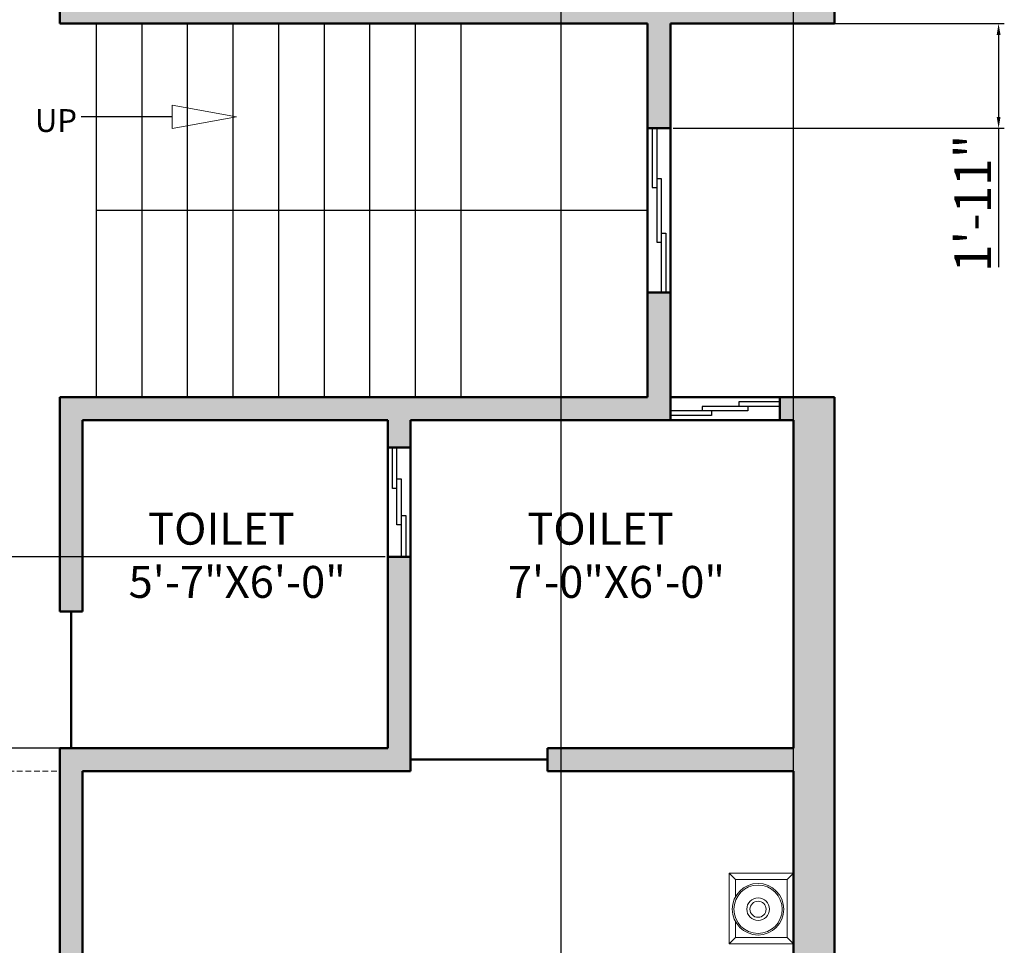
# Model space of a CAD drawing. Units: inches. Extents: x 1913 to 5309, y 1003 to 1733.
# Tile 20 of 23: x 4336 to 4552, y 1286 to 1489. Entities that reach past the tile are written whole.
import ezdxf

# ---------------------------------------------------------------- set-up
doc = ezdxf.new("R2010")
doc.units = ezdxf.units.IN
doc.linetypes.add('HIDDEN2', pattern=[0.1875, 0.125, -0.0625])
for name, color, linetype, lineweight in [('0.15', 34, 'Continuous', 15), ('A-ANNO-DIMS', 2, 'Continuous', 18), ('A-ANNO-SYMB', 1, 'Continuous', 18), ('A-ANNO-TEXT', 7, 'Continuous', 18), ('A-AREA-IDEN', 3, 'Continuous', 18), ('A-FLOR-PATT', 252, 'Continuous', 13), ('A-FLOR-STRS', 7, 'Continuous', 25), ('A-FURN', 8, 'Continuous', 18), ('A-GLAZ', 5, 'Continuous', 25), ('A-WALL', 7, 'Continuous', 50), ('A-WALL-OVHD', 8, 'HIDDEN2', 18)]:
    doc.layers.add(name, color=color, linetype=linetype, lineweight=lineweight)
doc.styles.get("Standard").update_dxf_attribs({"font": 'arial.ttf'})
doc.dimstyles.new('ISO-25', dxfattribs={"dimtxt": 8, "dimasz": 2.5, "dimexe": 1.25, "dimexo": 0.625, "dimtad": 1, "dimdec": 1, "dimlunit": 3, "dimtxsty": 'Standard', "dimcen": 2.5, "dimclrd": 256, "dimclrt": 1, "dimadec": 0, "dimazin": 0, "dimtfac": 1, "dimtdec": 1, "dimtmove": 0, "dimatfit": 3, "dimfxl": 1, "dimarcsym": 0})

# ---------------------------------------------------------------- blocks, each defined once
blk = doc.blocks.new('VELADOR')
at = {"layer": '0.15'}
for p, q in [((-0.2475, 0), (-0.2025, -0.045)), ((0.2475, 0), (0.2025, -0.045)), ((-0.2025, -0.405), (-0.2475, -0.45)), ((0.2475, -0.45), (0.2025, -0.405))]:
    blk.add_line(p, q, dxfattribs=at)
blk.add_lwpolyline([(-0.2475, 0), (-0.2475, -0.45), (0.2475, -0.45), (0.2475, 0)], close=True, dxfattribs=at)
blk.add_lwpolyline([(0.0921, -0.405), (0.2025, -0.405), (0.2025, -0.045), (-0.2025, -0.045), (-0.2025, -0.405), (-0.0818, -0.405)], dxfattribs=at)
for radius in [0.18, 0.1688, 0.0788, 0.0563]:
    blk.add_circle((0.0052, -0.2474), radius, dxfattribs=at)
blk = doc.blocks.new('WIN-24')
for p, q in [((0, 15), (0, 24)), ((1, 7), (1, 24)), ((2, 17), (1, 17)), ((2, 0), (2, 17)), ((1, 15), (0, 15)), ((3, 9), (2, 9)), ((3, 0), (3, 9)), ((2, 7), (1, 7))]:
    blk.add_line(p, q)
blk = doc.blocks.new('WIN-36')
for p, q in [((0, 23), (0, 36)), ((1, 11), (1, 36)), ((2, 25), (1, 25)), ((2, 0), (2, 25)), ((1, 23), (0, 23)), ((3, 13), (2, 13)), ((3, 0), (3, 13)), ((2, 11), (1, 11))]:
    blk.add_line(p, q)
blk = doc.blocks.new('*D110')
at = {"layer": 'A-ANNO-DIMS', "color": 0, "lineweight": -2, "transparency": 16777216}
for p, q in [((4479.84, 1487.96), (4552.46, 1487.96)), ((4479.84, 1464.96), (4552.46, 1464.96))]:
    blk.add_line(p, q, dxfattribs=at)
at = {"layer": 'A-ANNO-DIMS', "lineweight": -2, "transparency": 16777216}
for p, q in [((4551.21, 1485.46), (4551.21, 1467.46)), ((4551.21, 1464.96), (4551.21, 1434.49))]:
    blk.add_line(p, q, dxfattribs=at)
at = {"layer": 'A-ANNO-DIMS', "transparency": 16777216}
for points in [[(4550.8, 1485.46), (4551.63, 1485.46), (4551.21, 1487.96)], [(4550.8, 1467.46), (4551.63, 1467.46), (4551.21, 1464.96)]]:
    blk.add_solid(points, dxfattribs=at)
at = {"layer": 'Defpoints', "color": 0, "transparency": 16777216}
for p in [(4479.21, 1487.96), (4479.21, 1464.96), (4551.21, 1464.96)]:
    blk.add_point(p, dxfattribs=at)
at = {"layer": 'A-ANNO-DIMS', "color": 1, "transparency": 16777216, "insert": (4546.57, 1448.47), "char_height": 8, "attachment_point": 5, "rotation": 90}
blk.add_mtext('1\'-11"', dxfattribs=at)
blk = doc.blocks.new('*D113')
at = {"layer": 'A-ANNO-DIMS', "color": 0, "lineweight": -2, "transparency": 16777216}
for p, q in [((4455.21, 1180.59), (4455.21, 1724.21)), ((4506.21, 1180.59), (4506.21, 1724.21))]:
    blk.add_line(p, q, dxfattribs=at)
at = {"layer": 'A-ANNO-DIMS', "lineweight": -2, "transparency": 16777216}
blk.add_line((4457.71, 1722.96), (4503.71, 1722.96), dxfattribs=at)
at = {"layer": 'A-ANNO-DIMS', "transparency": 16777216}
for points in [[(4457.71, 1723.38), (4457.71, 1722.55), (4455.21, 1722.96)], [(4503.71, 1723.38), (4503.71, 1722.55), (4506.21, 1722.96)]]:
    blk.add_solid(points, dxfattribs=at)
at = {"layer": 'Defpoints', "color": 0, "transparency": 16777216}
for p in [(4506.21, 1722.96), (4455.21, 1179.96), (4506.21, 1179.96)]:
    blk.add_point(p, dxfattribs=at)
at = {"layer": 'A-ANNO-DIMS', "color": 1, "transparency": 16777216, "insert": (4480.71, 1727.68), "char_height": 8, "attachment_point": 5}
blk.add_mtext('4\'-3"', dxfattribs=at)
blk = doc.blocks.new('*D115')
at = {"layer": 'A-ANNO-DIMS', "color": 0, "lineweight": -2, "transparency": 16777216}
for p, q in [((4416.59, 1370.96), (3925.96, 1370.96)), ((4416.59, 1328.96), (3925.96, 1328.96))]:
    blk.add_line(p, q, dxfattribs=at)
at = {"layer": 'A-ANNO-DIMS', "lineweight": -2, "transparency": 16777216}
blk.add_line((3927.21, 1331.46), (3927.21, 1368.46), dxfattribs=at)
at = {"layer": 'A-ANNO-DIMS', "transparency": 16777216}
for points in [[(3926.8, 1368.46), (3927.63, 1368.46), (3927.21, 1370.96)], [(3926.8, 1331.46), (3927.63, 1331.46), (3927.21, 1328.96)]]:
    blk.add_solid(points, dxfattribs=at)
at = {"layer": 'Defpoints', "color": 0, "transparency": 16777216}
for p in [(3927.21, 1370.96), (4417.21, 1370.96), (4417.21, 1328.96)]:
    blk.add_point(p, dxfattribs=at)
at = {"layer": 'A-ANNO-DIMS', "color": 1, "transparency": 16777216, "insert": (3922.5, 1349.96), "char_height": 8, "attachment_point": 5, "rotation": 90}
blk.add_mtext('3\'-6"', dxfattribs=at)

msp = doc.modelspace()

# ---------------------------------------------------------------- hatches: boundary and pattern name
at = {"layer": 'A-FLOR-PATT'}
h = msp.add_hatch(color=256, dxfattribs=at)
h.dxf.hatch_style = 1
h.paths.add_polyline_path([(4179.21, 1155.93), (4164.35, 1155.93, -0.035946), (4163.9, 1155.96), (4161.21, 1155.96), (4161.21, 1173.96), (4152.21, 1173.96), (4152.21, 1146.96), (4179.21, 1146.96)])
h.paths.add_polyline_path([(4273.21, 1155.96), (4266.93, 1155.96), (4233.21, 1155.96), (4233.21, 1146.96), (4273.21, 1146.96)])
h.paths.add_polyline_path([(4285.21, 1328.96), (4152.21, 1328.96), (4152.21, 1305.96), (4161.21, 1305.96), (4161.21, 1323.96), (4285.21, 1323.96)])
h.paths.add_polyline_path([(4161.21, 1257.96), (4152.21, 1257.96), (4152.21, 1233.96), (4161.21, 1233.96), (4161.21, 1237.71)])
h.paths.add_polyline_path([(4515.21, 1405.96), (4503.21, 1405.96), (4503.21, 1400.96), (4506.21, 1400.96), (4506.21, 1328.96), (4452.21, 1328.96), (4452.21, 1323.96), (4506.21, 1323.96), (4506.21, 1179.96), (4455.21, 1179.96), (4455.21, 1170.96), (4515.21, 1170.96)])
h.paths.add_polyline_path([(4157.21, 1686.96), (3999.21, 1686.96), (3999.21, 1625.96), (4008.21, 1625.96), (4008.21, 1677.96), (4152.21, 1677.96), (4152.21, 1554.96), (4157.21, 1554.96), (4157.21, 1599.96), (4225.21, 1599.96), (4225.21, 1608.96), (4157.21, 1608.96)])
h.paths.add_polyline_path([(4008.21, 1513.96), (4157.21, 1513.96), (4157.21, 1518.96), (4008.21, 1518.96), (4008.21, 1571.96), (3999.21, 1571.96), (3999.21, 1420.96), (4050.21, 1420.96), (4050.21, 1429.96), (4008.21, 1429.96)])
h.paths.add_polyline_path([(4157.21, 1477.96), (4152.21, 1477.96), (4152.21, 1429.96), (4110.21, 1429.96), (4110.21, 1420.96), (4157.21, 1420.96)], flags=17)
h.paths.add_polyline_path([(4350.21, 1608.96), (4345.21, 1608.96), (4321.21, 1608.96), (4321.21, 1599.96), (4350.21, 1599.96)])
h.paths.add_polyline_path([(4515.21, 1686.96), (4345.21, 1686.96), (4345.21, 1644.96), (4350.21, 1644.96), (4350.21, 1677.96), (4506.21, 1677.96), (4506.21, 1557.96), (4423.21, 1557.96), (4423.21, 1552.96), (4506.21, 1552.96), (4506.21, 1492.96), (4428.21, 1492.96), (4428.21, 1522.96), (4423.21, 1522.96), (4423.21, 1492.96), (4345.21, 1492.96), (4345.21, 1487.96), (4474.21, 1487.96), (4474.21, 1464.96), (4479.21, 1464.96), (4479.21, 1487.96), (4515.21, 1487.96)])
h.paths.add_polyline_path([(4479.21, 1428.96), (4474.21, 1428.96), (4474.21, 1405.96), (4345.21, 1405.96), (4345.21, 1358.96), (4350.21, 1358.96), (4350.21, 1400.96), (4417.21, 1400.96), (4417.21, 1394.96), (4422.21, 1394.96), (4422.21, 1400.96), (4479.21, 1400.96)])
h.paths.add_polyline_path([(4350.21, 1323.96), (4422.21, 1323.96), (4422.21, 1370.96), (4417.21, 1370.96), (4417.21, 1328.96), (4345.21, 1328.96), (4345.21, 1158.97, -0.414214), (4342.21, 1155.96), (4327.21, 1155.96), (4327.21, 1146.96), (4350.21, 1146.96), (4350.21, 1170.96), (4401.21, 1170.96), (4401.21, 1179.96), (4350.21, 1179.96)])
h.paths.add_polyline_path([(4157.21, 1356.96), (4152.21, 1356.96), (4152.21, 1352.96), (4157.21, 1352.96)])
h.paths.add_polyline_path([(4157.21, 1396.96), (4152.21, 1396.96), (4152.21, 1392.96), (4157.21, 1392.96)])

# ---------------------------------------------------------------- linework, layer by layer
at = {"layer": 'A-ANNO-SYMB'}
msp.add_lwpolyline([(4384.04, 1467.46), (4369.88, 1470.02), (4369.88, 1464.91)], close=True, dxfattribs=at)
at = {"layer": 'A-FLOR-STRS'}
for p, q in [((4353.21, 1487.96), (4353.21, 1405.96)), ((4363.21, 1487.96), (4363.21, 1405.96)), ((4373.21, 1487.96), (4373.21, 1405.96)), ((4383.21, 1487.96), (4383.21, 1405.96)), ((4393.21, 1487.96), (4393.21, 1405.96)), ((4403.21, 1487.96), (4403.21, 1405.96)), ((4413.21, 1487.96), (4413.21, 1405.96)), ((4423.21, 1487.96), (4423.21, 1405.96)), ((4433.21, 1487.96), (4433.21, 1405.96)), ((4369.88, 1467.46), (4349.96, 1467.46)), ((4474.21, 1446.96), (4353.21, 1446.96))]:
    msp.add_line(p, q, dxfattribs=at)
at = {"layer": 'A-WALL'}
for p, q in [((4515.21, 1686.96), (4515.21, 1487.96)), ((4345.21, 1492.96), (4345.21, 1487.96)), ((4345.21, 1487.96), (4474.21, 1487.96)), ((4474.21, 1487.96), (4474.21, 1405.96)), ((4479.21, 1487.96), (4479.21, 1400.96)), ((4479.21, 1487.96), (4515.21, 1487.96)), ((4479.21, 1464.96), (4474.21, 1464.96)), ((4479.21, 1428.96), (4474.21, 1428.96)), ((4345.21, 1405.96), (4474.21, 1405.96)), ((4345.21, 1405.96), (4345.21, 1358.96)), ((4479.21, 1405.96), (4515.21, 1405.96)), ((4503.21, 1405.96), (4503.21, 1400.96)), ((4515.21, 1405.96), (4515.21, 1098.96)), ((4350.21, 1400.96), (4350.21, 1358.96)), ((4350.21, 1400.96), (4417.21, 1400.96)), ((4417.21, 1400.96), (4417.21, 1328.96)), ((4422.21, 1400.96), (4422.21, 1323.96)), ((4422.21, 1400.96), (4506.21, 1400.96)), ((4506.21, 1400.96), (4506.21, 1328.96)), ((4417.21, 1394.96), (4422.21, 1394.96)), ((4417.21, 1370.96), (4422.21, 1370.96)), ((4345.21, 1358.96), (4350.21, 1358.96)), ((4347.71, 1358.96), (4347.71, 1328.96)), ((4345.21, 1328.96), (4345.21, 1155.96)), ((4345.21, 1328.96), (4417.21, 1328.96)), ((4452.21, 1328.96), (4506.21, 1328.96)), ((4452.21, 1328.96), (4452.21, 1323.96)), ((4452.21, 1326.46), (4422.21, 1326.46)), ((4350.21, 1323.96), (4350.21, 1179.96)), ((4350.21, 1323.96), (4422.21, 1323.96)), ((4452.21, 1323.96), (4506.21, 1323.96)), ((4506.21, 1323.96), (4506.21, 1179.96))]:
    msp.add_line(p, q, dxfattribs=at)
at = {"layer": 'A-WALL-OVHD', "ltscale": 10}
for p, q in [((4285.21, 1328.96), (4345.21, 1328.96)), ((4285.21, 1323.96), (4345.21, 1323.96))]:
    msp.add_line(p, q, dxfattribs=at)

# ---------------------------------------------------------------- block references
at = {"layer": 'A-FURN', "xscale": 31.41542173157097, "yscale": 31.41542173157097, "zscale": 31.41542173157097, "rotation": 270}
msp.add_blockref('VELADOR', (4506.21, 1293.8), dxfattribs=at)
at = {"layer": 'A-GLAZ'}
for name, p, rotation in [('WIN-36', (4478.21, 1464.96), 180), ('WIN-24', (4503.21, 1401.96), 89.99999999999213)]:
    msp.add_blockref(name, p, dxfattribs=dict(at, rotation=rotation))
msp.add_blockref('WIN-24', (4418.21, 1370.96), dxfattribs=at)

# ---------------------------------------------------------------- texts
at = {"layer": 'A-ANNO-TEXT', "insert": (4339.77, 1469.16), "char_height": 5, "attachment_point": 1}
msp.add_mtext_dynamic_manual_height_columns('{UP}', width=10.7355, gutter_width=12.5, heights=[0], dxfattribs=at)
at = {"layer": 'A-AREA-IDEN', "char_height": 7, "attachment_point": 1}
for s, insert in [('  TOILET\\P5\'-7"X6\'-0"', (4360.33, 1380.62)), ('  TOILET\\P7\'-0"X6\'-0"', (4443.53, 1380.62))]:
    msp.add_mtext_dynamic_manual_height_columns(s, width=86.9528, gutter_width=12.5, heights=[0], dxfattribs=dict(at, insert=insert))

# ---------------------------------------------------------------- dimensions: what is measured, and where the dimension line sits
at = {"layer": 'A-ANNO-DIMS'}
dim = msp.add_linear_dim(base=(4506.21, 1722.96), p1=(4455.21, 1179.96), p2=(4506.21, 1179.96), dimstyle='ISO-25', override={"dimdec": 1, "dimlfac": 1, "dimrnd": 0, "dimzin": 1, "dimdsep": 46, "dimlunit": 4, "dimfrac": 2}, dxfattribs=at)
dim.commit()
dim.dimension.update_dxf_attribs({"geometry": '*D113', "text_midpoint": (4480.71, 1727.68)})
for base, p1, p2, picture, middle in [((4551.21, 1464.96), (4479.21, 1487.96), (4479.21, 1464.96), '*D110', (4546.57, 1448.47)), ((3927.21, 1370.96), (4417.21, 1328.96), (4417.21, 1370.96), '*D115', (3922.5, 1349.96))]:
    dim = msp.add_linear_dim(base=base, p1=p1, p2=p2, angle=90, dimstyle='ISO-25', override={"dimdec": 1, "dimlfac": 1, "dimrnd": 0, "dimzin": 1, "dimdsep": 46, "dimlunit": 4, "dimfrac": 2}, dxfattribs=at)
    dim.commit()
    dim.dimension.update_dxf_attribs({"geometry": picture, "text_midpoint": middle})

doc.saveas('drawing.dxf')
